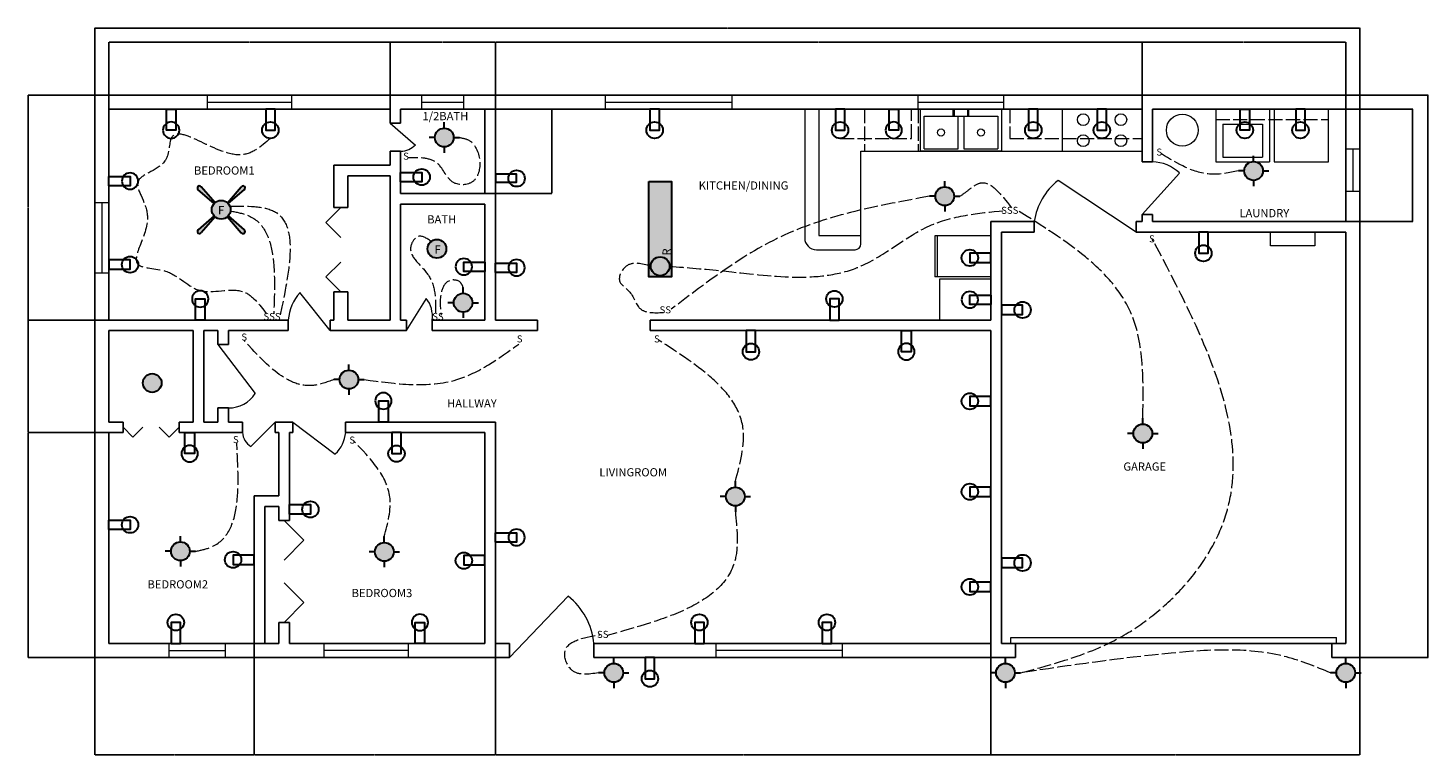
# Model space of a CAD drawing. Units: inches. Extents: x 2216 to 3412, y 979 to 1599.
import ezdxf

# ---------------------------------------------------------------- set-up
doc = ezdxf.new("R2010")
doc.units = ezdxf.units.IN
doc.linetypes.add('ACAD_ISO02W100', pattern=[15, 12, -3])
for name, color, linetype, lineweight in [('A-ANNO-DIMS', 2, 'Continuous', 18), ('A-AREA-IDEN', 7, 'Continuous', 18), ('A-DOOR', 7, 'Continuous', 18), ('A-EQPM', 9, 'Continuous', 18), ('A-FLOR-CASE', 9, 'Continuous', 18), ('A-FLOR-CASE-OVHD', 9, 'ACAD_ISO02W100', 13), ('A-FLOR-FIXT', 9, 'Continuous', 13), ('A-GLAZ', 40, 'Continuous', 18), ('A-WALL', 123, 'Continuous', 25), ('E-ANNO-IDEN', 7, 'Continuous', 18), ('E-FANS', 7, 'Continuous', 30), ('E-FANS-PATT', 32, 'Continuous', 13), ('E-LITE-CTRL', 9, 'ACAD_ISO02W100', 18), ('E-LITE-FIXT', 7, 'Continuous', 30), ('E-LITE-PATT', 51, 'Continuous', 13), ('E-LITE-SWCH', 7, 'Continuous', 30), ('E-POWR-RCPT', 40, 'Continuous', 30)]:
    doc.layers.add(name, color=color, linetype=linetype, lineweight=lineweight)
doc.styles.get("Standard").update_dxf_attribs({"font": 'arial.ttf'})
doc.dimstyles.get("Standard").update_dxf_attribs({"dimtxt": 0.18, "dimasz": 0.18, "dimexe": 0.18, "dimexo": 0.0625, "dimgap": 0.09, "dimtad": 0, "dimtih": 1, "dimtoh": 1, "dimdec": 4, "dimzin": 0, "dimdsep": 46, "dimtxsty": 'Standard', "dimcen": 0.09, "dimadec": 0, "dimazin": 0, "dimtfac": 1, "dimtdec": 4, "dimtofl": 0, "dimtmove": 0, "dimatfit": 3, "dimfxl": 1, "dimtolj": 1, "dimtzin": 0, "dimarcsym": 0})

# ---------------------------------------------------------------- blocks, each defined once
blk = doc.blocks.new('RECEPTACLE-WALL')
blk.add_lwpolyline([(-18, -4), (0, -4), (0, 4), (-18, 4)], close=True)
blk.add_circle((0, 0), 7)
blk = doc.blocks.new('LIGHT-ROUND-FOUR-TICKS')
h = blk.add_hatch(color=256)
h.dxf.hatch_style = 1
h.paths.add_polyline_path([(8, 0, 1), (-8, 0, 1)])
for p, q in [((0, 8), (0, 13)), ((-8, 0), (-13, 0)), ((8, 0), (13, 0)), ((0, -8), (0, -13))]:
    blk.add_line(p, q)
blk.add_circle((0, 0), 8)
blk = doc.blocks.new('WINDOW-72IN')
for p, q in [((-36, -6), (-36, 6)), ((-36, 0), (36, 0)), ((36, -6), (36, 6))]:
    blk.add_line(p, q)
blk = doc.blocks.new('WINDOW-36IN')
for p, q in [((-18, -6), (-18, 6)), ((-18, 0), (18, 0)), ((18, -6), (18, 6))]:
    blk.add_line(p, q)
blk = doc.blocks.new('WINDOW-108IN')
for p, q in [((-54, -6), (-54, 6)), ((-54, 0), (54, 0)), ((54, -6), (54, 6))]:
    blk.add_line(p, q)
blk = doc.blocks.new('DOOR-BIFOLD-48IN')
for p, q in [((17, 17), (0, 33.9)), ((0, 0), (17, 17))]:
    blk.add_line(p, q)
blk = doc.blocks.new('DOOR-BIFOLD-24IN')
for p, q in [((-8.5, -8.5), (-17, 0)), ((0, 0), (-8.5, -8.5))]:
    blk.add_line(p, q)
blk = doc.blocks.new('DOOR-BIFOLD-36IN')
for p, q in [((0, 0), (-12.7, -12.7)), ((-12.7, -12.7), (0, -25.5))]:
    blk.add_line(p, q)
blk = doc.blocks.new('*D9')
at = {"layer": 'A-ANNO-DIMS', "color": 0, "lineweight": -2, "transparency": 16777216}
for p, q in [((2273.5, 1542), (2273.5, 1599.1)), ((2273.7, 1598.9), (2813.2, 1598.9)), ((3353.3, 1598.9), (2813.9, 1598.9)), ((3353.5, 1542), (3353.5, 1599.1))]:
    blk.add_line(p, q, dxfattribs=at)
at = {"layer": 'A-ANNO-DIMS', "color": 0, "transparency": 16777216}
for points in [[(2273.7, 1598.9), (2273.7, 1598.8), (2273.5, 1598.9)], [(3353.3, 1598.9), (3353.3, 1598.8), (3353.5, 1598.9)]]:
    blk.add_solid(points, dxfattribs=at)
at = {"layer": 'Defpoints', "color": 0, "transparency": 16777216}
for p in [(3353.5, 1598.9), (2273.5, 1541.9), (3353.5, 1541.9)]:
    blk.add_point(p, dxfattribs=at)
at = {"layer": 'A-ANNO-DIMS', "color": 0, "transparency": 16777216, "insert": (2813.5, 1598.9), "char_height": 0.18, "attachment_point": 5}
blk.add_mtext('\\A1;1080', dxfattribs=at)
blk = doc.blocks.new('*D10')
at = {"layer": 'A-ANNO-DIMS', "color": 0, "lineweight": -2, "transparency": 16777216}
for p, q in [((3353.6, 1541.9), (3411.7, 1541.9)), ((3411.5, 1541.7), (3411.5, 1302.1)), ((3411.5, 1062.1), (3411.5, 1301.7)), ((3353.6, 1061.9), (3411.7, 1061.9))]:
    blk.add_line(p, q, dxfattribs=at)
at = {"layer": 'A-ANNO-DIMS', "color": 0, "transparency": 16777216}
for points in [[(3411.4, 1541.7), (3411.5, 1541.7), (3411.5, 1541.9)], [(3411.4, 1062.1), (3411.5, 1062.1), (3411.5, 1061.9)]]:
    blk.add_solid(points, dxfattribs=at)
at = {"layer": 'Defpoints', "color": 0, "transparency": 16777216}
for p in [(3353.5, 1541.9), (3411.5, 1541.9), (3353.5, 1061.9)]:
    blk.add_point(p, dxfattribs=at)
at = {"layer": 'A-ANNO-DIMS', "color": 0, "transparency": 16777216, "insert": (3411.5, 1301.9), "char_height": 0.18, "attachment_point": 5}
blk.add_mtext('\\A1;480', dxfattribs=at)
blk = doc.blocks.new('*D11')
at = {"layer": 'A-ANNO-DIMS', "color": 0, "lineweight": -2, "transparency": 16777216}
for p, q in [((2285.5, 1530), (2285.5, 1587.1)), ((2285.7, 1586.9), (2405.2, 1586.9)), ((2525.3, 1586.9), (2405.8, 1586.9)), ((2525.5, 1530), (2525.5, 1587.1))]:
    blk.add_line(p, q, dxfattribs=at)
at = {"layer": 'A-ANNO-DIMS', "color": 0, "transparency": 16777216}
for points in [[(2285.7, 1586.9), (2285.7, 1586.8), (2285.5, 1586.9)], [(2525.3, 1586.9), (2525.3, 1586.8), (2525.5, 1586.9)]]:
    blk.add_solid(points, dxfattribs=at)
at = {"layer": 'Defpoints', "color": 0, "transparency": 16777216}
for p in [(2525.5, 1586.9), (2285.5, 1529.9), (2525.5, 1529.9)]:
    blk.add_point(p, dxfattribs=at)
at = {"layer": 'A-ANNO-DIMS', "color": 0, "transparency": 16777216, "insert": (2405.5, 1586.9), "char_height": 0.18, "attachment_point": 5}
blk.add_mtext('\\A1;240', dxfattribs=at)
blk = doc.blocks.new('*D12')
at = {"layer": 'A-ANNO-DIMS', "color": 0, "lineweight": -2, "transparency": 16777216}
for p, q in [((2525.5, 1530), (2525.5, 1587.1)), ((2525.7, 1586.9), (2570.3, 1586.9)), ((2615.3, 1586.9), (2570.7, 1586.9)), ((2615.5, 1530), (2615.5, 1587.1))]:
    blk.add_line(p, q, dxfattribs=at)
at = {"layer": 'A-ANNO-DIMS', "color": 0, "transparency": 16777216}
for points in [[(2525.7, 1586.9), (2525.7, 1586.8), (2525.5, 1586.9)], [(2615.3, 1586.9), (2615.3, 1586.8), (2615.5, 1586.9)]]:
    blk.add_solid(points, dxfattribs=at)
at = {"layer": 'Defpoints', "color": 0, "transparency": 16777216}
for p in [(2615.5, 1586.9), (2525.5, 1529.9), (2615.5, 1529.9)]:
    blk.add_point(p, dxfattribs=at)
at = {"layer": 'A-ANNO-DIMS', "color": 0, "transparency": 16777216, "insert": (2570.5, 1586.9), "char_height": 0.18, "attachment_point": 5}
blk.add_mtext('\\A1;90', dxfattribs=at)
blk = doc.blocks.new('*D13')
at = {"layer": 'A-ANNO-DIMS', "color": 0, "lineweight": -2, "transparency": 16777216}
for p, q in [((2615.5, 1530), (2615.5, 1587.1)), ((2615.7, 1586.9), (2891.2, 1586.9)), ((3167.3, 1586.9), (2891.8, 1586.9)), ((3167.5, 1530), (3167.5, 1587.1))]:
    blk.add_line(p, q, dxfattribs=at)
at = {"layer": 'A-ANNO-DIMS', "color": 0, "transparency": 16777216}
for points in [[(2615.7, 1586.9), (2615.7, 1586.8), (2615.5, 1586.9)], [(3167.3, 1586.9), (3167.3, 1586.8), (3167.5, 1586.9)]]:
    blk.add_solid(points, dxfattribs=at)
at = {"layer": 'Defpoints', "color": 0, "transparency": 16777216}
for p in [(3167.5, 1586.9), (2615.5, 1529.9), (3167.5, 1529.9)]:
    blk.add_point(p, dxfattribs=at)
at = {"layer": 'A-ANNO-DIMS', "color": 0, "transparency": 16777216, "insert": (2891.5, 1586.9), "char_height": 0.18, "attachment_point": 5}
blk.add_mtext('\\A1;552', dxfattribs=at)
blk = doc.blocks.new('*D14')
at = {"layer": 'A-ANNO-DIMS', "color": 0, "lineweight": -2, "transparency": 16777216}
for p, q in [((3167.5, 1530), (3167.5, 1587.1)), ((3167.7, 1586.9), (3254.2, 1586.9)), ((3341.3, 1586.9), (3254.8, 1586.9)), ((3341.5, 1530), (3341.5, 1587.1))]:
    blk.add_line(p, q, dxfattribs=at)
at = {"layer": 'A-ANNO-DIMS', "color": 0, "transparency": 16777216}
for points in [[(3167.7, 1586.9), (3167.7, 1586.8), (3167.5, 1586.9)], [(3341.3, 1586.9), (3341.3, 1586.8), (3341.5, 1586.9)]]:
    blk.add_solid(points, dxfattribs=at)
at = {"layer": 'Defpoints', "color": 0, "transparency": 16777216}
for p in [(3341.5, 1586.9), (3167.5, 1529.9), (3341.5, 1529.9)]:
    blk.add_point(p, dxfattribs=at)
at = {"layer": 'A-ANNO-DIMS', "color": 0, "transparency": 16777216, "insert": (3254.5, 1586.9), "char_height": 0.18, "attachment_point": 5}
blk.add_mtext('\\A1;174', dxfattribs=at)
blk = doc.blocks.new('*D15')
at = {"layer": 'A-ANNO-DIMS', "color": 0, "lineweight": -2, "transparency": 16777216}
for p, q in [((2409.5, 1073.9), (2409.5, 978.8)), ((2273.5, 1061.9), (2273.5, 978.8)), ((2273.7, 979), (2341.2, 979)), ((2409.3, 979), (2341.8, 979))]:
    blk.add_line(p, q, dxfattribs=at)
at = {"layer": 'A-ANNO-DIMS', "color": 0, "transparency": 16777216}
for points in [[(2273.7, 979), (2273.7, 978.9), (2273.5, 979)], [(2409.3, 979), (2409.3, 978.9), (2409.5, 979)]]:
    blk.add_solid(points, dxfattribs=at)
at = {"layer": 'Defpoints', "color": 0, "transparency": 16777216}
for p in [(2409.5, 1073.9), (2273.5, 1061.9), (2409.5, 979)]:
    blk.add_point(p, dxfattribs=at)
at = {"layer": 'A-ANNO-DIMS', "color": 0, "transparency": 16777216, "insert": (2341.5, 979), "char_height": 0.18, "attachment_point": 5}
blk.add_mtext('\\A1;136', dxfattribs=at)
blk = doc.blocks.new('*D16')
at = {"layer": 'A-ANNO-DIMS', "color": 0, "lineweight": -2, "transparency": 16777216}
for p, q in [((2409.5, 1073.9), (2409.5, 978.8)), ((2615.5, 1073.9), (2615.5, 978.8)), ((2409.7, 979), (2512.2, 979)), ((2615.3, 979), (2512.8, 979))]:
    blk.add_line(p, q, dxfattribs=at)
at = {"layer": 'A-ANNO-DIMS', "color": 0, "transparency": 16777216}
for points in [[(2409.7, 979), (2409.7, 978.9), (2409.5, 979)], [(2615.3, 979), (2615.3, 978.9), (2615.5, 979)]]:
    blk.add_solid(points, dxfattribs=at)
at = {"layer": 'Defpoints', "color": 0, "transparency": 16777216}
for p in [(2409.5, 1073.9), (2615.5, 1073.9), (2615.5, 979)]:
    blk.add_point(p, dxfattribs=at)
at = {"layer": 'A-ANNO-DIMS', "color": 0, "transparency": 16777216, "insert": (2512.5, 979), "char_height": 0.18, "attachment_point": 5}
blk.add_mtext('\\A1;206', dxfattribs=at)
blk = doc.blocks.new('*D17')
at = {"layer": 'A-ANNO-DIMS', "color": 0, "lineweight": -2, "transparency": 16777216}
for p, q in [((2615.5, 1073.9), (2615.5, 978.8)), ((3038.5, 1073.9), (3038.5, 978.8)), ((2615.7, 979), (2826.7, 979)), ((3038.3, 979), (2827.3, 979))]:
    blk.add_line(p, q, dxfattribs=at)
at = {"layer": 'A-ANNO-DIMS', "color": 0, "transparency": 16777216}
for points in [[(2615.7, 979), (2615.7, 978.9), (2615.5, 979)], [(3038.3, 979), (3038.3, 978.9), (3038.5, 979)]]:
    blk.add_solid(points, dxfattribs=at)
at = {"layer": 'Defpoints', "color": 0, "transparency": 16777216}
for p in [(2615.5, 1073.9), (3038.5, 1073.9), (3038.5, 979)]:
    blk.add_point(p, dxfattribs=at)
at = {"layer": 'A-ANNO-DIMS', "color": 0, "transparency": 16777216, "insert": (2827, 979), "char_height": 0.18, "attachment_point": 5}
blk.add_mtext('\\A1;423', dxfattribs=at)
blk = doc.blocks.new('*D18')
at = {"layer": 'A-ANNO-DIMS', "color": 0, "lineweight": -2, "transparency": 16777216}
for p, q in [((3038.5, 1073.9), (3038.5, 978.8)), ((3353.5, 1061.9), (3353.5, 978.8)), ((3038.7, 979), (3195.7, 979)), ((3353.3, 979), (3196.3, 979))]:
    blk.add_line(p, q, dxfattribs=at)
at = {"layer": 'A-ANNO-DIMS', "color": 0, "transparency": 16777216}
for points in [[(3038.7, 979), (3038.7, 978.9), (3038.5, 979)], [(3353.3, 979), (3353.3, 978.9), (3353.5, 979)]]:
    blk.add_solid(points, dxfattribs=at)
at = {"layer": 'Defpoints', "color": 0, "transparency": 16777216}
for p in [(3038.5, 1073.9), (3353.5, 1061.9), (3353.5, 979)]:
    blk.add_point(p, dxfattribs=at)
at = {"layer": 'A-ANNO-DIMS', "color": 0, "transparency": 16777216, "insert": (3196, 979), "char_height": 0.18, "attachment_point": 5}
blk.add_mtext('\\A1;315', dxfattribs=at)
blk = doc.blocks.new('*D19')
at = {"layer": 'A-ANNO-DIMS', "color": 0, "lineweight": -2, "transparency": 16777216}
for p, q in [((2285.5, 1253.9), (2216.4, 1253.9)), ((2216.6, 1253.7), (2216.6, 1158.1)), ((2216.6, 1062.1), (2216.6, 1157.7)), ((2273.5, 1061.9), (2216.4, 1061.9))]:
    blk.add_line(p, q, dxfattribs=at)
at = {"layer": 'A-ANNO-DIMS', "color": 0, "transparency": 16777216}
for points in [[(2216.5, 1253.7), (2216.6, 1253.7), (2216.6, 1253.9)], [(2216.5, 1062.1), (2216.6, 1062.1), (2216.6, 1061.9)]]:
    blk.add_solid(points, dxfattribs=at)
at = {"layer": 'Defpoints', "color": 0, "transparency": 16777216}
for p in [(2216.6, 1253.9), (2285.5, 1253.9), (2273.5, 1061.9)]:
    blk.add_point(p, dxfattribs=at)
at = {"layer": 'A-ANNO-DIMS', "color": 0, "transparency": 16777216, "insert": (2216.6, 1157.9), "char_height": 0.18, "attachment_point": 5}
blk.add_mtext('\\A1;192', dxfattribs=at)
blk = doc.blocks.new('*D20')
at = {"layer": 'A-ANNO-DIMS', "color": 0, "lineweight": -2, "transparency": 16777216}
for p, q in [((2285.5, 1349.9), (2216.4, 1349.9)), ((2216.6, 1349.7), (2216.6, 1302.1)), ((2216.6, 1254.1), (2216.6, 1301.7)), ((2285.5, 1253.9), (2216.4, 1253.9))]:
    blk.add_line(p, q, dxfattribs=at)
at = {"layer": 'A-ANNO-DIMS', "color": 0, "transparency": 16777216}
for points in [[(2216.5, 1349.7), (2216.6, 1349.7), (2216.6, 1349.9)], [(2216.5, 1254.1), (2216.6, 1254.1), (2216.6, 1253.9)]]:
    blk.add_solid(points, dxfattribs=at)
at = {"layer": 'Defpoints', "color": 0, "transparency": 16777216}
for p in [(2216.6, 1349.9), (2285.5, 1349.9), (2285.5, 1253.9)]:
    blk.add_point(p, dxfattribs=at)
at = {"layer": 'A-ANNO-DIMS', "color": 0, "transparency": 16777216, "insert": (2216.6, 1301.9), "char_height": 0.18, "attachment_point": 5}
blk.add_mtext('\\A1;96', dxfattribs=at)
blk = doc.blocks.new('*D21')
at = {"layer": 'A-ANNO-DIMS', "color": 0, "lineweight": -2, "transparency": 16777216}
for p, q in [((2273.5, 1541.9), (2216.4, 1541.9)), ((2216.6, 1541.7), (2216.6, 1446.1)), ((2216.6, 1350.1), (2216.6, 1445.7)), ((2285.5, 1349.9), (2216.4, 1349.9))]:
    blk.add_line(p, q, dxfattribs=at)
at = {"layer": 'A-ANNO-DIMS', "color": 0, "transparency": 16777216}
for points in [[(2216.5, 1541.7), (2216.6, 1541.7), (2216.6, 1541.9)], [(2216.5, 1350.1), (2216.6, 1350.1), (2216.6, 1349.9)]]:
    blk.add_solid(points, dxfattribs=at)
at = {"layer": 'Defpoints', "color": 0, "transparency": 16777216}
for p in [(2216.6, 1541.9), (2273.5, 1541.9), (2285.5, 1349.9)]:
    blk.add_point(p, dxfattribs=at)
at = {"layer": 'A-ANNO-DIMS', "color": 0, "transparency": 16777216, "insert": (2216.6, 1445.9), "char_height": 0.18, "attachment_point": 5}
blk.add_mtext('\\A1;192', dxfattribs=at)
blk = doc.blocks.new('*D22')
at = {"layer": 'A-ANNO-DIMS', "color": 0, "lineweight": -2, "transparency": 16777216}
for p, q in [((3341.6, 1529.9), (3398.7, 1529.9)), ((3398.5, 1529.7), (3398.5, 1482.1)), ((3398.5, 1434.1), (3398.5, 1481.7)), ((3341.6, 1433.9), (3398.7, 1433.9))]:
    blk.add_line(p, q, dxfattribs=at)
at = {"layer": 'A-ANNO-DIMS', "color": 0, "transparency": 16777216}
for points in [[(3398.4, 1529.7), (3398.5, 1529.7), (3398.5, 1529.9)], [(3398.4, 1434.1), (3398.5, 1434.1), (3398.5, 1433.9)]]:
    blk.add_solid(points, dxfattribs=at)
at = {"layer": 'Defpoints', "color": 0, "transparency": 16777216}
for p in [(3341.5, 1529.9), (3341.5, 1433.9), (3398.5, 1433.9)]:
    blk.add_point(p, dxfattribs=at)
at = {"layer": 'A-ANNO-DIMS', "color": 0, "transparency": 16777216, "insert": (3398.5, 1481.9), "char_height": 0.18, "attachment_point": 5}
blk.add_mtext('\\A1;96', dxfattribs=at)
blk = doc.blocks.new('*D23')
at = {"layer": 'A-ANNO-DIMS', "color": 0, "lineweight": -2, "transparency": 16777216}
for p, q in [((2606.6, 1529.9), (2663.7, 1529.9)), ((2663.5, 1529.7), (2663.5, 1494.1)), ((2663.5, 1458.1), (2663.5, 1493.7)), ((2606.6, 1457.9), (2663.7, 1457.9))]:
    blk.add_line(p, q, dxfattribs=at)
at = {"layer": 'A-ANNO-DIMS', "color": 0, "transparency": 16777216}
for points in [[(2663.4, 1529.7), (2663.5, 1529.7), (2663.5, 1529.9)], [(2663.4, 1458.1), (2663.5, 1458.1), (2663.5, 1457.9)]]:
    blk.add_solid(points, dxfattribs=at)
at = {"layer": 'Defpoints', "color": 0, "transparency": 16777216}
for p in [(2606.5, 1529.9), (2606.5, 1457.9), (2663.5, 1457.9)]:
    blk.add_point(p, dxfattribs=at)
at = {"layer": 'A-ANNO-DIMS', "color": 0, "transparency": 16777216, "insert": (2663.5, 1493.9), "char_height": 0.18, "attachment_point": 5}
blk.add_mtext('\\A1;72', dxfattribs=at)

msp = doc.modelspace()

# ---------------------------------------------------------------- hatches: boundary and pattern name
at = {"layer": 'E-FANS-PATT'}
h = msp.add_hatch(color=256, dxfattribs=at)
h.dxf.hatch_style = 1
h.paths.add_polyline_path([(2364.3, 1463.6, 1.185008), (2361.7, 1461), (2375.3, 1449.2, -0.034921), (2376.1, 1450)])
h = msp.add_hatch(color=256, dxfattribs=at)
h.dxf.hatch_style = 1
h.paths.add_polyline_path([(2401, 1461, 1.185008), (2398.4, 1463.6), (2386.6, 1450, -0.034921), (2387.4, 1449.2)])
h = msp.add_hatch(color=256, dxfattribs=at)
h.dxf.hatch_style = 1
h.paths.add_polyline_path([(2373.3, 1444, 1), (2389.3, 1444, 1)])
h = msp.add_hatch(color=256, dxfattribs=at)
h.dxf.hatch_style = 1
h.paths.add_polyline_path([(2375.3, 1438.7), (2361.7, 1426.9, 1.185008), (2364.3, 1424.4), (2376.1, 1437.9, -0.034921)])
h = msp.add_hatch(color=256, dxfattribs=at)
h.dxf.hatch_style = 1
h.paths.add_polyline_path([(2387.4, 1438.7, -0.034921), (2386.6, 1437.9), (2398.4, 1424.4, 1.185008), (2401, 1426.9)])
h = msp.add_hatch(color=256, dxfattribs=at)
h.dxf.hatch_style = 1
h.paths.add_polyline_path([(2557.5, 1410.7, 1), (2573.5, 1410.7, 1)])
at = {"layer": 'E-LITE-PATT'}
h = msp.add_hatch(color=256, dxfattribs=at)
h.dxf.hatch_style = 1
h.paths.add_polyline_path([(3270.8, 1477.1, 0.361905), (3264.2, 1484.9), (3261.3, 1484.9, 0.361905), (3254.8, 1477.1, 1)])
h = msp.add_hatch(color=256, dxfattribs=at)
h.dxf.hatch_style = 1
h.paths.add_polyline_path([(2764.2, 1395.8, 1), (2748.1, 1395.8, 1)], flags=0)
h.paths.add_polyline_path([(2765.7, 1468), (2746.5, 1468), (2746.5, 1386.9), (2765.7, 1386.9)])
h.paths.add_polyline_path([(2764.2, 1395.8, -1), (2748.1, 1395.8, -1)], flags=16)
h = msp.add_hatch(color=256, dxfattribs=at)
h.dxf.hatch_style = 1
h.paths.add_polyline_path([(2764.2, 1395.8, 1), (2748.1, 1395.8, 1)])
h = msp.add_hatch(color=256, dxfattribs=at)
h.dxf.hatch_style = 1
h.paths.add_polyline_path([(2330.4, 1296.2, 1), (2314.4, 1296.2, 1)])

# ---------------------------------------------------------------- linework, layer by layer
at = {"layer": 'A-DOOR'}
for p, q in [((2525.5, 1517.9), (2547.2, 1499.2)), ((3167.5, 1439.9), (3199.5, 1475.3)), ((3162.5, 1424.9), (3095.8, 1468.9)), ((2474.5, 1340.9), (2448.6, 1373.5)), ((2539.5, 1340.9), (2556.5, 1368.4)), ((2378.5, 1328.9), (2410.4, 1287.2)), ((2427.5, 1262.9), (2406.7, 1242.1)), ((2442.5, 1262.9), (2478.7, 1235.6)), ((2627.5, 1061.9), (2677.5, 1114.3)), ((3055.5, 1073.9), (3055.5, 1078.9)), ((3055.5, 1078.9), (3333.5, 1078.9)), ((3333.5, 1073.9), (3333.5, 1078.9)), ((3059.5, 1073.9), (3055.5, 1073.9)), ((3329.5, 1073.9), (3333.5, 1073.9))]:
    msp.add_line(p, q, dxfattribs=at)
for centre, radius, start, end in [((2534.4, 1512.1), 18.1, 270.4688, 314.998), ((3175.2, 1449.5), 35.5, 46.7549, 87.8857), ((3128.5, 1426.5), 53.5, 127.6704, 172.0354), ((2477, 1347.4), 38.5, 137.3873, 176.1961), ((2535.5, 1352.7), 26.2, 353.8877, 36.8476), ((2387.5, 1302.4), 27.5, 269.9904, 326.5059), ((2414.1, 1254.7), 14.6, 183.0521, 239.6493), ((2459.2, 1256.4), 28.5, 313.254, 355.0664), ((2640.8, 1068), 59.1, 5.7197, 51.5233)]:
    msp.add_arc(centre, radius, start, end, dxfattribs=at)
at = {"layer": 'A-EQPM'}
for p, q in [((3326.7, 1529.9), (3230.4, 1529.9)), ((3230.4, 1529.9), (3230.4, 1484.9)), ((3276.4, 1529.9), (3276.4, 1484.9)), ((3280.4, 1529.9), (3280.4, 1484.9)), ((3326.7, 1484.9), (3326.7, 1529.9)), ((3236.4, 1516.9), (3236.4, 1488.9)), ((3236.4, 1516.9), (3270.4, 1516.9)), ((3270.4, 1516.9), (3270.4, 1488.9)), ((3230.4, 1484.9), (3276.4, 1484.9)), ((3236.4, 1488.9), (3270.4, 1488.9)), ((3280.4, 1484.9), (3326.7, 1484.9))]:
    msp.add_line(p, q, dxfattribs=at)
msp.add_lwpolyline([(3277.3, 1424.9), (3315.2, 1424.9), (3315.2, 1413.2), (3277.3, 1413.2)], close=True, dxfattribs=at)
for centre, radius in [((3117.3, 1520.9), 5), ((3149.5, 1520.9), 5), ((3201.9, 1511.9), 13.6), ((3117.3, 1502.9), 5), ((3149.5, 1502.9), 5)]:
    msp.add_circle(centre, radius, dxfattribs=at)
at = {"layer": 'A-FLOR-CASE'}
for p, q in [((2891.5, 1529.9), (2879.5, 1529.9)), ((2879.5, 1529.9), (2879.5, 1419.9)), ((2891.5, 1529.9), (2891.5, 1421.9)), ((2978.4, 1493.9), (2978.4, 1529.9)), ((3047.5, 1529.9), (3047.5, 1493.9)), ((3099.3, 1529.9), (3099.3, 1493.9)), ((2927.5, 1421.9), (2927.5, 1493.9)), ((2927.5, 1493.9), (3167.5, 1493.9)), ((3047.5, 1493.9), (2978.4, 1493.9)), ((2891.5, 1421.9), (2927.5, 1421.9)), ((2927.5, 1414.9), (2927.5, 1421.9)), ((3038.5, 1421.7), (2990.6, 1421.7)), ((2990.6, 1421.7), (2990.6, 1386.7)), ((2992.6, 1421.7), (2992.6, 1386.7)), ((2889.5, 1409.9), (2922.5, 1409.9)), ((3038.5, 1386.7), (2990.6, 1386.7)), ((3038.5, 1384.7), (2994.6, 1384.7)), ((2994.6, 1384.7), (2994.6, 1349.9)), ((2990.6, 1349.9), (3038.5, 1349.9))]:
    msp.add_line(p, q, dxfattribs=at)
for centre, radius, start, end in [((2889.5, 1419.9), 10, 180, 270), ((2922.5, 1414.9), 5, 270, 0)]:
    msp.add_arc(centre, radius, start, end, dxfattribs=at)
at = {"layer": 'A-FLOR-CASE-OVHD'}
for p, q in [((2930.5, 1529.9), (2930.5, 1493.9)), ((2970.6, 1504.9), (2970.6, 1529.9)), ((2976.4, 1529.9), (2976.4, 1493.9)), ((3054.6, 1529.9), (3054.6, 1504.9)), ((3230.4, 1520.9), (3326.7, 1520.9)), ((2909.7, 1504.9), (2970.6, 1504.9)), ((3054.6, 1504.9), (3167.5, 1504.9))]:
    msp.add_line(p, q, dxfattribs=at)
at = {"layer": 'A-FLOR-FIXT'}
for p, q in [((2981.4, 1529.9), (3044.5, 1529.9)), ((2981.4, 1495.9), (2981.4, 1523.9)), ((2981.4, 1523.9), (3044.5, 1523.9)), ((3006.4, 1523.9), (3006.4, 1529.9)), ((3007.4, 1523.9), (3007.4, 1529.9)), ((3010.4, 1495.9), (3010.4, 1523.9)), ((3015.5, 1523.9), (3015.5, 1495.9)), ((3018.5, 1529.9), (3018.5, 1523.9)), ((3019.5, 1529.9), (3019.5, 1523.9)), ((3044.5, 1523.9), (3044.5, 1495.9)), ((2981.4, 1495.9), (3010.4, 1495.9)), ((3015.5, 1495.9), (3044.5, 1495.9))]:
    msp.add_line(p, q, dxfattribs=at)
for centre in [(2995.9, 1509.9), (3030, 1509.9)]:
    msp.add_circle(centre, 3, dxfattribs=at)
at = {"layer": 'A-GLAZ'}
for p, q in [((2976.4, 1529.9), (2976.4, 1541.9)), ((2976.4, 1535.9), (3049.5, 1535.9)), ((3049.5, 1529.9), (3049.5, 1541.9)), ((2285.5, 1449.9), (2273.5, 1449.9)), ((2279.5, 1449.9), (2279.5, 1389.9)), ((2285.5, 1389.9), (2273.5, 1389.9)), ((2336.7, 1073.9), (2336.7, 1061.9)), ((2336.7, 1067.9), (2384.7, 1067.9)), ((2384.7, 1073.9), (2384.7, 1061.9))]:
    msp.add_line(p, q, dxfattribs=at)
at = {"layer": 'A-WALL'}
for p, q in [((2285.5, 1529.9), (2525.5, 1529.9)), ((2285.5, 1349.9), (2285.5, 1529.9)), ((2525.5, 1517.9), (2525.5, 1529.9)), ((2534.5, 1517.9), (2534.5, 1529.9)), ((2534.5, 1529.9), (2606.5, 1529.9)), ((2606.5, 1457.9), (2606.5, 1529.9)), ((2615.5, 1349.9), (2615.5, 1529.9)), ((2615.5, 1529.9), (3167.5, 1529.9)), ((3167.5, 1493.9), (3167.5, 1529.9)), ((3176.5, 1493.9), (3176.5, 1529.9)), ((3176.5, 1529.9), (3341.5, 1529.9)), ((3341.5, 1529.9), (3341.5, 1433.9)), ((2525.5, 1517.9), (2534.5, 1517.9)), ((2525.5, 1493.9), (2534.5, 1493.9)), ((2525.5, 1493.9), (2525.5, 1481.9)), ((2525.5, 1481.9), (2525.5, 1493.9)), ((2534.5, 1457.9), (2534.5, 1493.9)), ((3167.5, 1493.9), (3167.5, 1484.9)), ((3167.5, 1484.9), (3176.5, 1484.9)), ((3176.5, 1493.9), (3176.5, 1484.9)), ((2525.5, 1481.9), (2477.5, 1481.9)), ((2477.5, 1481.9), (2477.5, 1445.9)), ((2489.5, 1445.9), (2489.5, 1472.9)), ((2489.5, 1472.9), (2525.5, 1472.9)), ((2525.5, 1349.9), (2525.5, 1472.9)), ((2534.5, 1457.9), (2606.5, 1457.9)), ((2534.5, 1448.9), (2606.5, 1448.9)), ((2534.5, 1349.9), (2534.5, 1448.9)), ((2606.5, 1349.9), (2606.5, 1448.9)), ((2477.5, 1445.9), (2489.5, 1445.9)), ((3167.5, 1433.9), (3167.5, 1439.9)), ((3167.5, 1439.9), (3176.5, 1439.9)), ((3176.5, 1433.9), (3176.5, 1439.9)), ((3038.5, 1433.9), (3075.5, 1433.9)), ((3038.5, 1349.9), (3038.5, 1433.9)), ((3047.5, 1073.9), (3047.5, 1424.9)), ((3047.5, 1424.9), (3075.5, 1424.9)), ((3075.5, 1424.9), (3075.5, 1433.9)), ((3162.5, 1424.9), (3162.5, 1433.9)), ((3162.5, 1433.9), (3167.5, 1433.9)), ((3162.5, 1424.9), (3341.5, 1424.9)), ((3176.5, 1433.9), (3341.5, 1433.9)), ((3341.5, 1424.9), (3341.5, 1073.9)), ((2489.5, 1373.9), (2477.5, 1373.9)), ((2477.5, 1373.9), (2477.5, 1349.9)), ((2489.5, 1349.9), (2489.5, 1373.9)), ((2285.5, 1349.9), (2438.5, 1349.9)), ((2285.5, 1340.9), (2357.5, 1340.9)), ((2285.5, 1262.9), (2285.5, 1340.9)), ((2357.5, 1262.9), (2357.5, 1340.9)), ((2366.5, 1262.9), (2366.5, 1340.9)), ((2366.5, 1340.9), (2378.5, 1340.9)), ((2378.5, 1328.9), (2378.5, 1340.9)), ((2387.5, 1328.9), (2387.5, 1340.9)), ((2387.5, 1340.9), (2438.5, 1340.9)), ((2438.5, 1349.9), (2438.5, 1340.9)), ((2474.5, 1349.9), (2474.5, 1340.9)), ((2474.5, 1349.9), (2477.5, 1349.9)), ((2474.5, 1340.9), (2539.5, 1340.9)), ((2525.5, 1349.9), (2489.5, 1349.9)), ((2489.5, 1349.9), (2525.5, 1349.9)), ((2534.5, 1349.9), (2539.5, 1349.9)), ((2539.5, 1340.9), (2539.5, 1349.9)), ((2561.5, 1340.9), (2561.5, 1349.9)), ((2561.5, 1349.9), (2606.5, 1349.9)), ((2561.5, 1340.9), (2651.5, 1340.9)), ((2615.5, 1349.9), (2651.5, 1349.9)), ((2651.5, 1340.9), (2651.5, 1349.9)), ((2747.5, 1340.9), (2747.5, 1349.9)), ((2747.5, 1349.9), (3038.5, 1349.9)), ((2747.5, 1340.9), (3038.5, 1340.9)), ((3038.5, 1073.9), (3038.5, 1340.9)), ((2378.5, 1328.9), (2387.5, 1328.9)), ((2378.5, 1262.9), (2378.5, 1274.9)), ((2387.5, 1274.9), (2378.5, 1274.9)), ((2387.5, 1262.9), (2387.5, 1274.9)), ((2297.5, 1262.9), (2285.5, 1262.9)), ((2297.5, 1253.9), (2297.5, 1262.9)), ((2345.5, 1253.9), (2345.5, 1262.9)), ((2357.5, 1262.9), (2345.5, 1262.9)), ((2378.5, 1262.9), (2366.5, 1262.9)), ((2399.5, 1262.9), (2387.5, 1262.9)), ((2399.5, 1253.9), (2399.5, 1262.9)), ((2427.5, 1253.9), (2427.5, 1262.9)), ((2442.5, 1262.9), (2427.5, 1262.9)), ((2442.5, 1253.9), (2442.5, 1262.9)), ((2615.5, 1262.9), (2487.5, 1262.9)), ((2487.5, 1253.9), (2487.5, 1262.9)), ((2615.5, 1073.9), (2615.5, 1262.9)), ((2285.5, 1073.9), (2285.5, 1253.9)), ((2297.5, 1253.9), (2285.5, 1253.9)), ((2399.5, 1253.9), (2345.5, 1253.9)), ((2430.5, 1253.9), (2427.5, 1253.9)), ((2430.5, 1199.9), (2430.5, 1253.9)), ((2442.5, 1253.9), (2439.5, 1253.9)), ((2439.5, 1178.9), (2439.5, 1253.9)), ((2606.5, 1253.9), (2487.5, 1253.9)), ((2606.5, 1073.9), (2606.5, 1253.9)), ((2430.5, 1199.9), (2409.5, 1199.9)), ((2409.5, 1199.9), (2409.5, 1073.9)), ((2430.5, 1190.9), (2418.5, 1190.9)), ((2418.5, 1190.9), (2418.5, 1073.9)), ((2430.5, 1178.9), (2430.5, 1190.9)), ((2439.5, 1178.9), (2430.5, 1178.9)), ((2430.5, 1073.9), (2430.5, 1091.9)), ((2439.5, 1091.9), (2430.5, 1091.9)), ((2439.5, 1073.9), (2439.5, 1091.9)), ((2430.5, 1073.9), (2285.5, 1073.9)), ((2606.5, 1073.9), (2439.5, 1073.9)), ((2627.5, 1073.9), (2615.5, 1073.9)), ((2627.5, 1073.9), (2627.5, 1061.9)), ((2699.5, 1073.9), (2699.5, 1061.9)), ((3038.5, 1073.9), (2699.5, 1073.9)), ((3341.5, 1073.9), (3047.5, 1073.9)), ((3059.5, 1073.9), (3059.5, 1061.9)), ((3329.5, 1073.9), (3329.5, 1061.9))]:
    msp.add_line(p, q, dxfattribs=at)
for points in [[(2627.5, 1061.9), (2273.5, 1061.9), (2273.5, 1541.9), (3353.5, 1541.9), (3353.5, 1061.9), (3329.5, 1061.9)], [(3059.5, 1061.9), (2699.5, 1061.9)]]:
    msp.add_lwpolyline(points, dxfattribs=at)
at = {"layer": 'E-FANS'}
for p, q in [((2375.3, 1449.2), (2361.7, 1461)), ((2376.1, 1450), (2364.3, 1463.6)), ((2386.6, 1450), (2398.4, 1463.6)), ((2387.4, 1449.2), (2401, 1461)), ((2375.3, 1438.7), (2361.7, 1426.9)), ((2376.1, 1437.9), (2364.3, 1424.4)), ((2386.6, 1437.9), (2398.4, 1424.4)), ((2387.4, 1438.7), (2401, 1426.9))]:
    msp.add_line(p, q, dxfattribs=at)
for centre in [(2381.3, 1444), (2565.5, 1410.7)]:
    msp.add_circle(centre, 8, dxfattribs=at)
for centre, start, end in [((2362.8, 1462.5), 35.3204, 234.6796), ((2399.9, 1462.5), 305.3204, 144.6796), ((2362.8, 1425.4), 125.3204, 324.6796), ((2399.9, 1425.4), 215.3204, 54.6796)]:
    msp.add_arc(centre, 1.84, start, end, dxfattribs=at)
at = {"layer": 'E-LITE-CTRL'}
for points, knots in [([(2423.3, 1504.9), (2415.3, 1497.9), (2391.4, 1476.9), (2334.7, 1527.1), (2338.3, 1479.2), (2298.2, 1472.4), (2331, 1436.1), (2294.6, 1392.8), (2340.8, 1395), (2360.8, 1366.8), (2399.9, 1382.2), (2413.9, 1363.4), (2420, 1355.2)], [0, 0, 0, 0, 30.047406, 89.863093, 108.951457, 138.376427, 168.139973, 211.337932, 235.3272, 269.252947, 305.241446, 333.405225, 333.405225, 333.405225, 333.405225]), ([(2584.8, 1505.6), (2587.7, 1505.1), (2602.5, 1502.5), (2606.9, 1465.2), (2575.5, 1464.2), (2568.2, 1488.9), (2550.7, 1488.5), (2541.1, 1488.2)], [0, 0, 0, 0, 8.662284, 43.783378, 60.267429, 81.179957, 106.922964, 106.922964, 106.922964, 106.922964]), ([(3249.8, 1477.1), (3241.9, 1475.5), (3218.8, 1470.8), (3198, 1483.3), (3184.2, 1491.6)], [0, 0, 0, 0, 23.460511, 69.144582, 69.144582, 69.144582, 69.144582]), ([(3012.1, 1455.5), (3014.6, 1457.2), (3019.6, 1460.9), (3035, 1473.5), (3046.8, 1457.7), (3056.1, 1445.5)], [0, 0, 0, 0, 9.1234, 19.084524, 54.164029, 54.164029, 54.164029, 54.164029]), ([(2388.7, 1447), (2403.2, 1447.2), (2451.3, 1447.7), (2439.7, 1392.4), (2431.6, 1353.8)], [0, 0, 0, 0, 38.35097, 127.034252, 127.034252, 127.034252, 127.034252]), ([(2986.1, 1455.5), (2943.3, 1447.7), (2862, 1432.9), (2796.6, 1382.8), (2765.6, 1359.1)], [0, 0, 0, 0, 128.56351, 243.723209, 243.723209, 243.723209, 243.723209]), ([(2389.3, 1442.9), (2394.3, 1442), (2429.1, 1435.7), (2427.5, 1392.4), (2426.2, 1355.3)], [0, 0, 0, 0, 14.841617, 101.859812, 101.859812, 101.859812, 101.859812]), ([(2764.2, 1395.8), (2779.2, 1394.6), (2833.1, 1390.4), (2917, 1376.5), (2982.7, 1436.8), (3027.6, 1441.1), (3049.6, 1443.3)], [0, 0, 0, 0, 45.825249, 163.81909, 231.439206, 296.3434, 296.3434, 296.3434, 296.3434]), ([(3168.2, 1266.1), (3168.8, 1297.8), (3170.1, 1375.5), (3102.1, 1417.9), (3061.8, 1443)], [0, 0, 0, 0, 89.646771, 220.17598, 220.17598, 220.17598, 220.17598]), ([(2560.6, 1417), (2556.6, 1419.7), (2549.4, 1424.5), (2537.4, 1406.3), (2564.6, 1389), (2564.5, 1367.6), (2564.4, 1355.9)], [0, 0, 0, 0, 12.138826, 21.911932, 50.034928, 83.83465, 83.83465, 83.83465, 83.83465]), ([(3063.9, 1048.9), (3092.8, 1056.6), (3164.4, 1075.5), (3287.7, 1207.6), (3220.3, 1335.5), (3176.3, 1419)], [0, 0, 0, 0, 89.682029, 222.193393, 471.275218, 471.275218, 471.275218, 471.275218]), ([(2748.1, 1395.8), (2740.6, 1398), (2728, 1401.6), (2717.7, 1382.4), (2732.8, 1374.5), (2736.6, 1355.6), (2751, 1356), (2758.7, 1356.3)], [0, 0, 0, 0, 20.893414, 34.704822, 46.391935, 64.098889, 84.10713, 84.10713, 84.10713, 84.10713]), ([(2587.9, 1377.7), (2587.2, 1379.5), (2585.2, 1384.3), (2573.6, 1384.8), (2567.2, 1370.9), (2568.4, 1360.7), (2569.1, 1354.2)], [0, 0, 0, 0, 5.390898, 15.005628, 26.281089, 45.822214, 45.822214, 45.822214, 45.822214]), ([(2477.4, 1299.1), (2471.5, 1296.9), (2442.7, 1286.5), (2419.4, 1312.2), (2400.8, 1332.7)], [0, 0, 0, 0, 18.007133, 88.603661, 88.603661, 88.603661, 88.603661]), ([(2503.4, 1299.1), (2530.7, 1295.4), (2579.1, 1288.8), (2618.2, 1317), (2635.3, 1329.3)], [0, 0, 0, 0, 79.055371, 139.97603, 139.97603, 139.97603, 139.97603]), ([(2820.3, 1212.3), (2824.4, 1227.7), (2838.1, 1279), (2789.1, 1310.6), (2754.7, 1332.8)], [0, 0, 0, 0, 44.894821, 149.870276, 149.870276, 149.870276, 149.870276]), ([(2359.5, 1152.6), (2363.8, 1153.5), (2399.1, 1160.8), (2396.7, 1205.6), (2394.6, 1244.9)], [0, 0, 0, 0, 12.794169, 104.738359, 104.738359, 104.738359, 104.738359]), ([(2520.6, 1165.1), (2523.6, 1176.6), (2531.7, 1207.6), (2508.8, 1231.7), (2494.4, 1246.9)], [0, 0, 0, 0, 33.882305, 91.153952, 91.153952, 91.153952, 91.153952]), ([(2820.3, 1186.3), (2821.7, 1172.2), (2827.4, 1113), (2761.2, 1094.7), (2710.8, 1080.8)], [0, 0, 0, 0, 40.012019, 167.604034, 167.604034, 167.604034, 167.604034]), ([(2703.5, 1048.9), (2694.8, 1047.6), (2680.3, 1045.4), (2668.9, 1074.9), (2690.1, 1078.8), (2704.5, 1081.4)], [0, 0, 0, 0, 23.073561, 38.815881, 72.462281, 72.462281, 72.462281, 72.462281]), ([(3328.5, 1048.9), (3316.1, 1054), (3273, 1071.5), (3181, 1066.3), (3106.3, 1055.2), (3063.9, 1048.9)], [0, 0, 0, 0, 40.115082, 138.553031, 268.144978, 268.144978, 268.144978, 268.144978])]:
    msp.add_open_spline(points, degree=3, knots=knots, dxfattribs=at)
at = {"layer": 'E-LITE-FIXT'}
for p, q in [((3262.8, 1485.1), (3262.8, 1490.1)), ((3254.8, 1477.1), (3249.8, 1477.1)), ((3270.8, 1477.1), (3275.8, 1477.1)), ((3262.8, 1469.1), (3262.8, 1464.1))]:
    msp.add_line(p, q, dxfattribs=at)
msp.add_lwpolyline([(2746.5, 1468), (2765.7, 1468), (2765.7, 1386.9), (2746.5, 1386.9)], close=True, dxfattribs=at)
for centre, radius in [((3262.8, 1477.1), 8), ((2756.1, 1395.8), 8.04), ((2322.4, 1296.2), 8)]:
    msp.add_circle(centre, radius, dxfattribs=at)
at = {"layer": 'E-POWR-RCPT'}
for points in [[(3251.2, 1529.9), (3259.2, 1529.9), (3259.2, 1511.9), (3251.2, 1511.9)], [(2534.5, 1475.9), (2552.5, 1475.9), (2552.5, 1467.9), (2534.5, 1467.9)], [(2615.5, 1467.4), (2633.5, 1467.4), (2633.5, 1474.4), (2615.5, 1474.4)], [(2439.5, 1192.4), (2457.5, 1192.4), (2457.5, 1184.4), (2439.5, 1184.4)], [(2285.5, 1179.2), (2303.5, 1179.2), (2303.5, 1171.2), (2285.5, 1171.2)], [(2606.5, 1149), (2588.5, 1149), (2588.5, 1141), (2606.5, 1141)]]:
    msp.add_lwpolyline(points, close=True, dxfattribs=at)
for centre in [(3255.3, 1511.9), (2552.5, 1471.9), (2633.5, 1470.7), (2457.5, 1188.3), (2303.5, 1175.2), (2588.5, 1144.6)]:
    msp.add_circle(centre, 7, dxfattribs=at)

# ---------------------------------------------------------------- block references
at = {"layer": 'A-DOOR'}
for name, p in [('DOOR-BIFOLD-36IN', (2483.5, 1445.9)), ('DOOR-BIFOLD-36IN', (2483.5, 1399.4)), ('DOOR-BIFOLD-24IN', (2314.5, 1258.4)), ('DOOR-BIFOLD-24IN', (2345.5, 1258.4)), ('DOOR-BIFOLD-48IN', (2435, 1145)), ('DOOR-BIFOLD-48IN', (2435, 1091.9))]:
    msp.add_blockref(name, p, dxfattribs=at)
at = {"layer": 'A-GLAZ'}
for name, p in [('WINDOW-72IN', (2405.5, 1535.9)), ('WINDOW-36IN', (2570.5, 1535.9)), ('WINDOW-108IN', (2763.5, 1535.9))]:
    msp.add_blockref(name, p, dxfattribs=at)
for name, p, rotation in [('WINDOW-36IN', (3347.5, 1477.9), 270.0000000000009), ('WINDOW-72IN', (2505, 1067.9), 180), ('WINDOW-108IN', (2857.5, 1067.9), 180)]:
    msp.add_blockref(name, p, dxfattribs=dict(at, rotation=rotation))
at = {"layer": 'E-LITE-FIXT'}
for p in [(2571.8, 1505.6), (2999.1, 1455.5), (2587.9, 1364.7), (2490.4, 1299.1), (3168.2, 1253.1), (2820.3, 1199.3), (2520.6, 1152.1), (3341.5, 1048.9)]:
    msp.add_blockref('LIGHT-ROUND-FOUR-TICKS', p, dxfattribs=at)
at = {"layer": 'E-LITE-FIXT', "rotation": 180}
for p in [(2346.5, 1152.6), (2716.5, 1048.9), (3050.9, 1048.9)]:
    msp.add_blockref('LIGHT-ROUND-FOUR-TICKS', p, dxfattribs=at)
at = {"layer": 'E-POWR-RCPT', "extrusion": (0, 0, -1), "zscale": -1}
for p, rotation in [((-2338.6, 1511.9), 270.0000000000025), ((-2955.5, 1511.9), 270.0000000000025), ((-2303.5, 1468.5), 180), ((-2633.5, 1394.5), 180), ((-2363.4, 1367.9), 89.99999999999788), ((-2966.3, 1322.9), 270), ((-2519.8, 1280.9), 90.0000000000021), ((-2354.4, 1235.9), 270), ((-2633.5, 1164.4), 180), ((-2551, 1091.9), 90)]:
    msp.add_blockref('RECEPTACLE-WALL', p, dxfattribs=dict(at, rotation=rotation))
at = {"layer": 'E-POWR-RCPT'}
for p, rotation in [((2423.3, 1511.9), 270.0000000000005), ((2751.4, 1511.9), 270.0000000000005), ((2909.7, 1511.9), 270.0000000000025), ((3074.7, 1511.9), 270.0000000000005), ((3133.2, 1511.9), 270.0000000000025), ((3302.8, 1511.9), 269.9999999999984), ((3219.9, 1406.9), 269.9999999999984), ((3020.5, 1403), 180), ((2904.9, 1367.9), 90.00000000000003), ((2833.6, 1322.9), 270), ((3020.5, 1280.6), 180), ((2531, 1235.9), 270.0000000000021), ((3020.5, 1203.4), 180), ((2391.5, 1145.4), 180), ((3020.5, 1122.2), 180), ((2342.6, 1091.9), 90.0000000000021), ((2789.6, 1091.9), 90.00000000000423), ((2898.5, 1091.9), 90.0000000000021), ((2747.4, 1043.9), 270.0000000000021)]:
    msp.add_blockref('RECEPTACLE-WALL', p, dxfattribs=dict(at, rotation=rotation))
for p in [(2303.5, 1397.2), (3065.5, 1358.5), (3065.5, 1142.7)]:
    msp.add_blockref('RECEPTACLE-WALL', p, dxfattribs=at)
at = {"layer": 'E-POWR-RCPT', "extrusion": (0, 0, -1), "zscale": -1}
for p in [(-2588.5, 1395.4), (-3020.5, 1367.2)]:
    msp.add_blockref('RECEPTACLE-WALL', p, dxfattribs=at)

# ---------------------------------------------------------------- texts
at = {"layer": 'A-AREA-IDEN'}
for tag, p in [('1/2BATH', (2553.2, 1520.4)), ('BEDROOM1', (2358.1, 1474)), ('KITCHEN/DINING', (2789, 1461.2)), ('BATH', (2557.2, 1432.3)), ('LAUNDRY', (3250.7, 1437.6)), ('HALLWAY', (2574.2, 1275.3)), ('LIVINGROOM', (2704.2, 1216.5)), ('GARAGE', (3151.6, 1221.4)), ('BEDROOM2', (2318.4, 1120.9)), ('BEDROOM3', (2492.7, 1113.5))]:
    msp.add_attdef(tag, p, '', height=7, dxfattribs=at)
at = {"layer": 'E-ANNO-IDEN'}
for p in [(2378.6, 1440.1), (2563.5, 1406.5)]:
    msp.add_attdef('F', p, '', height=7, dxfattribs=at)
msp.add_attdef('R', (2765.1, 1404.9), '', height=7, rotation=90, dxfattribs=at)
at = {"layer": 'E-LITE-SWCH'}
for tag, p in [('S', (3179.8, 1490.2)), ('S', (2536.7, 1486.7)), ('SSS', (3047.3, 1440.5)), ('S', (3173.5, 1416.2)), ('SSS', (2417.4, 1349.9)), ('SS', (2561.5, 1349.9)), ('SS', (2755.6, 1355.6)), ('S', (2398.5, 1332.4)), ('S', (2633.7, 1330.8)), ('S', (2750.9, 1330.8)), ('S', (2391.4, 1244.9)), ('S', (2490.7, 1244.5)), ('SS', (2702.2, 1078.7))]:
    msp.add_attdef(tag, p, '', height=6, dxfattribs=at)

# ---------------------------------------------------------------- dimensions: what is measured, and where the dimension line sits
at = {"layer": 'A-ANNO-DIMS'}
for base, p1, p2, picture, middle in [((3353.5, 1598.9), (2273.5, 1541.9), (3353.5, 1541.9), '*D9', (2813.5, 1598.9)), ((2525.5, 1586.9), (2285.5, 1529.9), (2525.5, 1529.9), '*D11', (2405.5, 1586.9)), ((2615.5, 1586.9), (2525.5, 1529.9), (2615.5, 1529.9), '*D12', (2570.5, 1586.9)), ((3167.5, 1586.9), (2615.5, 1529.9), (3167.5, 1529.9), '*D13', (2891.5, 1586.9)), ((3341.5, 1586.9), (3167.5, 1529.9), (3341.5, 1529.9), '*D14', (3254.5, 1586.9)), ((2409.5, 979), (2273.5, 1061.9), (2409.5, 1073.9), '*D15', (2341.5, 979)), ((2615.5, 979), (2409.5, 1073.9), (2615.5, 1073.9), '*D16', (2512.5, 979)), ((3038.5, 979), (2615.5, 1073.9), (3038.5, 1073.9), '*D17', (2827, 979)), ((3353.5, 979), (3038.5, 1073.9), (3353.5, 1061.9), '*D18', (3196, 979))]:
    dim = msp.add_linear_dim(base=base, p1=p1, p2=p2, dimstyle='Standard', override={"dimdec": 0, "dimlfac": 1, "dimrnd": 0, "dimzin": 0, "dimdsep": 46, "dimlunit": 2}, dxfattribs=at)
    dim.commit()
    dim.dimension.update_dxf_attribs({"geometry": picture, "text_midpoint": middle})
for base, p1, p2, angle, picture, middle in [((2216.6, 1541.9), (2285.5, 1349.9), (2273.5, 1541.9), 90, '*D21', (2216.6, 1445.9)), ((3411.5, 1541.9), (3353.5, 1061.9), (3353.5, 1541.9), 90, '*D10', (3411.5, 1301.9)), ((2663.5, 1457.9), (2606.5, 1529.9), (2606.5, 1457.9), 270, '*D23', (2663.5, 1493.9)), ((3398.5, 1433.9), (3341.5, 1529.9), (3341.5, 1433.9), 270, '*D22', (3398.5, 1481.9)), ((2216.6, 1349.9), (2285.5, 1253.9), (2285.5, 1349.9), 90, '*D20', (2216.6, 1301.9)), ((2216.6, 1253.9), (2273.5, 1061.9), (2285.5, 1253.9), 90, '*D19', (2216.6, 1157.9))]:
    dim = msp.add_linear_dim(base=base, p1=p1, p2=p2, angle=angle, dimstyle='Standard', override={"dimdec": 0, "dimlfac": 1, "dimrnd": 0, "dimzin": 0, "dimdsep": 46, "dimlunit": 2}, dxfattribs=at)
    dim.commit()
    dim.dimension.update_dxf_attribs({"geometry": picture, "text_midpoint": middle})

doc.saveas('drawing.dxf')
